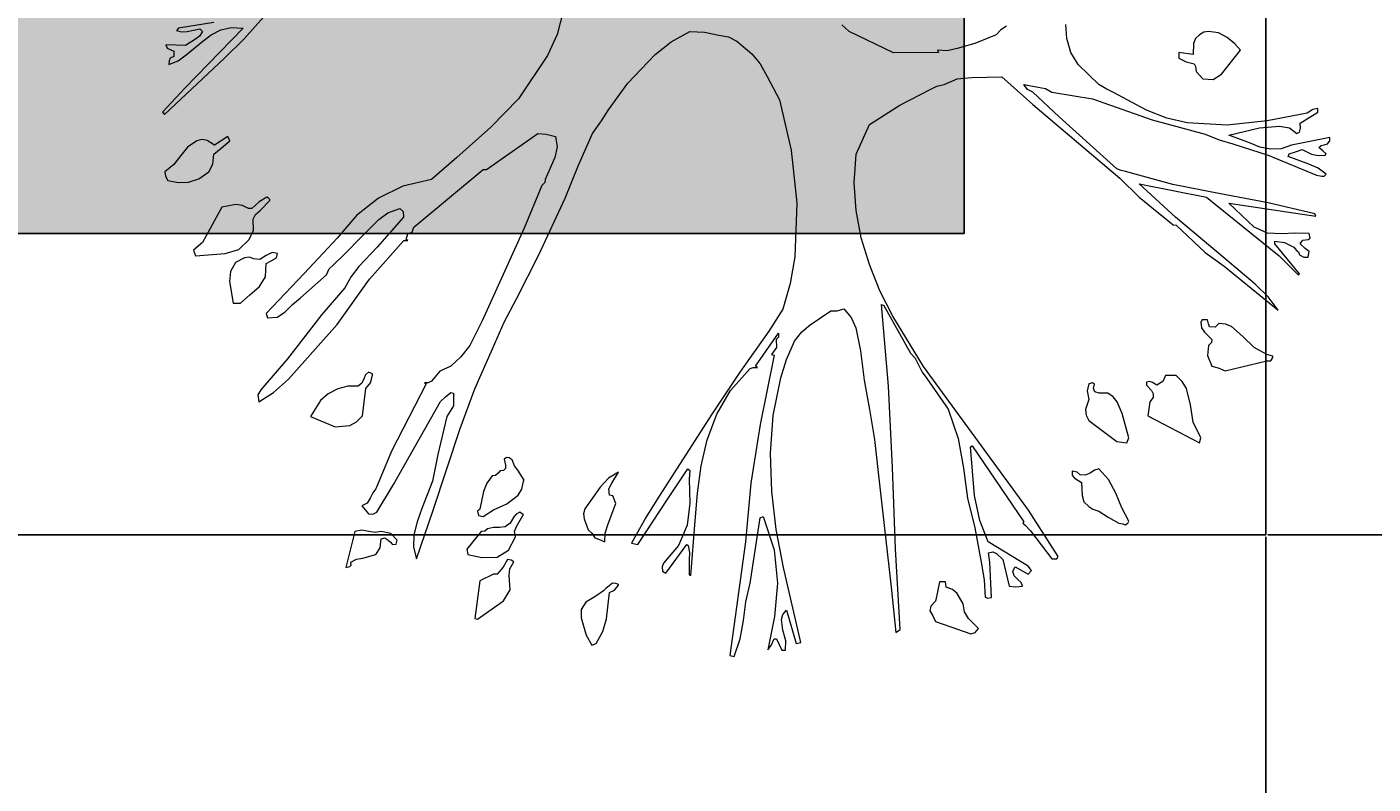
# Model space of a CAD drawing. Units: inches. Extents: x 84 to 1044, y -280 to 906.
# Tile 43 of 105: x 955 to 995, y -129 to -107. Entities that reach past the tile are written whole.
import ezdxf

# ---------------------------------------------------------------- set-up
doc = ezdxf.new("R2010")
doc.units = ezdxf.units.IN
for name, color, linetype, lineweight in [('A-ANNO-DIMS', 2, 'Continuous', 18), ('C-PROP', 7, 'Continuous', 25), ('L-PLNT', 114, 'Continuous', 15)]:
    doc.layers.add(name, color=color, linetype=linetype, lineweight=lineweight)
doc.layers.add('L-PLNT-PATT', color=9, linetype='Continuous', lineweight=9, true_color=0xafd9aa)
doc.styles.get("Standard").update_dxf_attribs({"font": 'arial.ttf'})
doc.dimstyles.get("Standard").update_dxf_attribs({"dimtxt": 0.18, "dimasz": 0.18, "dimexe": 0.18, "dimexo": 0.0625, "dimgap": 0.09, "dimtad": 0, "dimtih": 1, "dimtoh": 1, "dimdec": 4, "dimzin": 0, "dimdsep": 46, "dimtxsty": 'Standard', "dimcen": 0.09, "dimadec": 0, "dimazin": 0, "dimtfac": 1, "dimtdec": 4, "dimtofl": 0, "dimtmove": 0, "dimatfit": 3, "dimfxl": 1, "dimtolj": 1, "dimtzin": 0, "dimarcsym": 0})

# ---------------------------------------------------------------- blocks, each defined once
blk = doc.blocks.new('A$C37E508DF')
for p, q in [((0.9287, 0.7825), (0.936, 0.7542)), ((1.3151, 0.7487), (1.2919, 0.7752)), ((1.352, 0.7684), (1.3948, 0.7615)), ((0.1153, 0.7427), (0.1244, 0.7504)), ((0.1244, 0.7504), (0.1351, 0.7559)), ((0.1351, 0.7559), (0.1471, 0.7577)), ((0.1471, 0.7577), (0.1527, 0.7568)), ((0.1527, 0.7568), (0.1578, 0.7538)), ((0.1578, 0.7538), (0.1629, 0.7491)), ((0.3186, 0.7491), (0.3199, 0.7662)), ((0.3919, 0.7641), (0.3988, 0.7598)), ((0.3988, 0.7598), (0.4043, 0.7538)), ((0.4043, 0.7538), (0.4301, 0.7431)), ((0.5287, 0.7319), (0.5823, 0.7577)), ((0.5823, 0.7577), (0.5913, 0.7658)), ((0.7285, 0.7512), (0.7182, 0.7461)), ((0.7401, 0.7534), (0.7285, 0.7512)), ((0.7577, 0.7568), (0.7401, 0.7534)), ((0.7752, 0.7577), (0.7577, 0.7568)), ((0.798, 0.7452), (0.7752, 0.7577)), ((0.936, 0.7542), (0.9476, 0.7285)), ((1.3309, 0.7624), (1.3164, 0.7615)), ((1.3164, 0.7615), (1.3871, 0.6891)), ((1.3434, 0.7598), (1.3309, 0.7624)), ((1.355, 0.7538), (1.3434, 0.7598)), ((1.3653, 0.7461), (1.355, 0.7538)), ((1.3687, 0.7607), (1.3657, 0.7577)), ((1.3657, 0.7577), (1.3691, 0.7521)), ((1.3841, 0.7577), (1.3687, 0.7607)), ((1.3691, 0.7521), (1.3743, 0.7482)), ((1.3914, 0.7572), (1.3841, 0.7577)), ((1.397, 0.759), (1.3914, 0.7572)), ((1.3948, 0.7615), (1.397, 0.759)), ((0.1081, 0.7349), (0.1153, 0.7427)), ((0.1312, 0.7058), (0.1081, 0.7349)), ((0.1629, 0.7491), (0.1651, 0.7431)), ((0.1651, 0.7431), (0.1655, 0.7298)), ((0.3139, 0.7324), (0.3186, 0.7491)), ((0.4301, 0.7431), (0.4515, 0.7371)), ((0.4515, 0.7371), (0.4635, 0.7341)), ((0.4635, 0.7341), (0.4755, 0.7349)), ((0.4755, 0.7349), (0.4742, 0.7324)), ((0.7182, 0.7461), (0.7002, 0.7307)), ((0.8173, 0.7298), (0.798, 0.7452)), ((1.3391, 0.7255), (1.3151, 0.7487)), ((1.3854, 0.7294), (1.3653, 0.7461)), ((1.3743, 0.7482), (1.3863, 0.7405)), ((1.3863, 0.7405), (1.4099, 0.7414)), ((1.4086, 0.7375), (1.4004, 0.7337)), ((1.4099, 0.7414), (1.4086, 0.7375)), ((0.1646, 0.7186), (0.1629, 0.7152)), ((0.1741, 0.7208), (0.1646, 0.7186)), ((0.1655, 0.7298), (0.1831, 0.7324)), ((0.1831, 0.7255), (0.1741, 0.7208)), ((0.1831, 0.7324), (0.1831, 0.7255)), ((0.28, 0.6933), (0.3049, 0.7178)), ((0.3049, 0.7178), (0.3139, 0.7324)), ((0.4742, 0.7324), (0.5287, 0.7319)), ((0.6903, 0.7186), (0.6818, 0.7032)), ((0.7002, 0.7307), (0.6903, 0.7186)), ((0.8344, 0.7122), (0.8173, 0.7298)), ((0.9476, 0.7285), (0.9828, 0.6762)), ((1.4116, 0.6569), (1.3391, 0.7255)), ((1.3953, 0.7221), (1.3854, 0.7294)), ((1.4064, 0.7178), (1.3953, 0.7221)), ((1.4004, 0.7337), (1.4004, 0.7272)), ((1.4004, 0.7272), (1.4047, 0.7255)), ((1.4047, 0.7255), (1.406, 0.7221)), ((1.406, 0.7221), (1.4064, 0.7178)), ((0.1415, 0.6994), (0.1312, 0.7058)), ((0.1621, 0.7092), (0.1539, 0.7002)), ((0.1629, 0.7152), (0.1621, 0.7092)), ((0.3975, 0.7028), (0.3598, 0.6693)), ((0.4339, 0.7019), (0.3975, 0.7028)), ((0.4515, 0.7002), (0.4339, 0.7019)), ((0.6818, 0.7032), (0.6667, 0.6749)), ((0.8503, 0.6951), (0.8344, 0.7122)), ((0.1539, 0.7002), (0.1415, 0.6994)), ((0.262, 0.6839), (0.271, 0.6882)), ((0.271, 0.6882), (0.28, 0.6933)), ((0.3443, 0.6886), (0.337, 0.6843)), ((0.3533, 0.6903), (0.3443, 0.6886)), ((0.3709, 0.6933), (0.3533, 0.6903)), ((0.3598, 0.6843), (0.3662, 0.6873)), ((0.3662, 0.6873), (0.3709, 0.6933)), ((0.4674, 0.6933), (0.4515, 0.7002)), ((0.476, 0.6912), (0.4674, 0.6933)), ((0.4832, 0.6878), (0.476, 0.6912)), ((0.521, 0.6685), (0.4832, 0.6878)), ((0.8739, 0.6629), (0.8503, 0.6951)), ((1.3871, 0.6891), (1.4141, 0.6599)), ((0.2877, 0.6762), (0.2152, 0.6505)), ((0.2221, 0.6625), (0.262, 0.6839)), ((0.3598, 0.6693), (0.2543, 0.5797)), ((0.337, 0.6843), (0.2877, 0.6762)), ((0.328, 0.6543), (0.3598, 0.6843)), ((0.6667, 0.6749), (0.6526, 0.614)), ((0.9828, 0.6762), (1.0162, 0.6415)), ((0.0146, 0.6599), (0.0146, 0.6642)), ((0.0146, 0.6642), (0.0206, 0.6633)), ((0.036, 0.6466), (0.0146, 0.6599)), ((0.0206, 0.6633), (0.0274, 0.6586)), ((0.0274, 0.6586), (0.0759, 0.6492)), ((0.1728, 0.647), (0.1977, 0.6526)), ((0.1977, 0.6526), (0.2221, 0.6625)), ((0.2581, 0.5913), (0.328, 0.6543)), ((0.5578, 0.6449), (0.521, 0.6685)), ((0.8824, 0.6492), (0.8739, 0.6629)), ((1.4141, 0.6599), (1.4116, 0.6569)), ((0.0356, 0.6406), (0.036, 0.6466)), ((0.0369, 0.6355), (0.0356, 0.6406)), ((0.0489, 0.641), (0.0399, 0.6342)), ((0.0609, 0.6428), (0.0489, 0.641)), ((0.0853, 0.641), (0.0609, 0.6428)), ((0.0759, 0.6492), (0.1244, 0.644)), ((0.1226, 0.632), (0.0853, 0.641)), ((0.1244, 0.644), (0.1728, 0.647)), ((0.2152, 0.6505), (0.1509, 0.6333)), ((0.5737, 0.6089), (0.5578, 0.6449)), ((0.8932, 0.6342), (0.8824, 0.6492)), ((1.0162, 0.6415), (1.0574, 0.605)), ((0, 0.629), (0.0467, 0.62)), ((0, 0.6252), (0, 0.629)), ((0.003, 0.6213), (0, 0.6252)), ((0.0069, 0.6204), (0.003, 0.6213)), ((0.0107, 0.6196), (0.0069, 0.6204)), ((0.0399, 0.6342), (0.0369, 0.6355)), ((0.0467, 0.62), (0.0592, 0.6153)), ((0.1175, 0.6213), (0.0746, 0.6076)), ((0.0849, 0.6175), (0.0973, 0.6226)), ((0.0973, 0.6226), (0.1226, 0.632)), ((0.1342, 0.6265), (0.1175, 0.6213)), ((0.1509, 0.6333), (0.1342, 0.6265)), ((0.9103, 0.5956), (0.8932, 0.6342)), ((0.9382, 0.6303), (0.936, 0.6179)), ((0.9493, 0.6333), (0.9382, 0.6303)), ((0.9596, 0.6342), (0.9493, 0.6333)), ((1.0218, 0.5904), (0.9596, 0.6342)), ((1.3327, 0.6252), (1.3348, 0.6303)), ((1.343, 0.6162), (1.3327, 0.6252)), ((1.3348, 0.6303), (1.3511, 0.62)), ((1.3511, 0.62), (1.3601, 0.6256)), ((1.3601, 0.6256), (1.3661, 0.6269)), ((1.3661, 0.6269), (1.3725, 0.6252)), ((1.3725, 0.6252), (1.3837, 0.6175)), ((0.0047, 0.6093), (0.0086, 0.6132)), ((0.0056, 0.6076), (0.0047, 0.6093)), ((0.0141, 0.6072), (0.0056, 0.6076)), ((0.0086, 0.6132), (0.0133, 0.617)), ((0.0133, 0.617), (0.0107, 0.6196)), ((0.0223, 0.6089), (0.0141, 0.6072)), ((0.0746, 0.6076), (0.0163, 0.5836)), ((0.0334, 0.6145), (0.0223, 0.6089)), ((0.0257, 0.5969), (0.0506, 0.6063)), ((0.0416, 0.6119), (0.0334, 0.6145)), ((0.0493, 0.6093), (0.0416, 0.6119)), ((0.0506, 0.6063), (0.0493, 0.6093)), ((0.0592, 0.6153), (0.072, 0.6149)), ((0.072, 0.6149), (0.0849, 0.6175)), ((0.5763, 0.5741), (0.5737, 0.6089)), ((0.6526, 0.614), (0.6457, 0.5497)), ((0.936, 0.6179), (0.939, 0.605)), ((0.939, 0.605), (0.9506, 0.5784)), ((1.0574, 0.605), (1.0883, 0.5784)), ((1.352, 0.6089), (1.343, 0.6162)), ((1.3533, 0.5969), (1.352, 0.6089)), ((1.3837, 0.6175), (1.3918, 0.6072)), ((1.3918, 0.6072), (1.4004, 0.5964)), ((0.0047, 0.5849), (0.0141, 0.5921)), ((0.0141, 0.5921), (0.0257, 0.5969)), ((0.1904, 0.5724), (0.2474, 0.5879)), ((0.2474, 0.5879), (0.253, 0.5892)), ((0.253, 0.5892), (0.2581, 0.5913)), ((0.9262, 0.5557), (0.9103, 0.5956)), ((1.0256, 0.5904), (1.0218, 0.5904)), ((1.1097, 0.5205), (1.0256, 0.5904)), ((1.358, 0.5874), (1.3533, 0.5969)), ((1.37, 0.5789), (1.358, 0.5874)), ((1.4004, 0.5964), (1.4111, 0.5874)), ((1.4111, 0.5874), (1.4103, 0.5823)), ((0.0069, 0.5823), (0.0047, 0.5849)), ((0.0099, 0.5823), (0.0069, 0.5823)), ((0.0163, 0.5836), (0.0099, 0.5823)), ((0.1325, 0.5608), (0.1904, 0.5724)), ((0.2311, 0.5729), (0.1496, 0.557)), ((0.1869, 0.5325), (0.2311, 0.5729)), ((0.2543, 0.5797), (0.2311, 0.557)), ((0.5737, 0.5407), (0.5763, 0.5741)), ((0.9506, 0.5784), (0.951, 0.5746)), ((0.951, 0.5746), (0.9545, 0.5711)), ((0.9545, 0.5711), (0.9759, 0.5193)), ((1.0883, 0.5784), (1.123, 0.5703)), ((1.3824, 0.575), (1.37, 0.5789)), ((1.3953, 0.5746), (1.3824, 0.575)), ((1.4077, 0.5771), (1.3953, 0.5746)), ((1.4103, 0.5823), (1.4077, 0.5771)), ((0.1496, 0.557), (0.0613, 0.4858)), ((0.0746, 0.5501), (0.1325, 0.5608)), ((0.2311, 0.557), (0.1899, 0.5235)), ((0.9583, 0.4871), (0.9262, 0.5557)), ((1.123, 0.5703), (1.1526, 0.5557)), ((1.1526, 0.5557), (1.1792, 0.5347)), ((1.2842, 0.554), (1.2855, 0.5557)), ((1.2855, 0.5557), (1.2876, 0.557)), ((1.2876, 0.557), (1.2971, 0.551)), ((0.1226, 0.5497), (0.0171, 0.5338)), ((0.0184, 0.5368), (0.0746, 0.5501)), ((0.0917, 0.5205), (0.1226, 0.5497)), ((0.5677, 0.5077), (0.5737, 0.5407)), ((0.6457, 0.5497), (0.6483, 0.4845)), ((1.1226, 0.5394), (1.1221, 0.5325)), ((1.1268, 0.5433), (1.1226, 0.5394)), ((1.141, 0.5377), (1.1268, 0.5433)), ((1.2842, 0.5527), (1.2842, 0.554)), ((1.2958, 0.5407), (1.2842, 0.5527)), ((1.3014, 0.536), (1.2958, 0.5407)), ((1.2971, 0.551), (1.3057, 0.5433)), ((1.3057, 0.5433), (1.3099, 0.5433)), ((1.3099, 0.5433), (1.3172, 0.5467)), ((1.3172, 0.5467), (1.3254, 0.548)), ((1.3254, 0.548), (1.3421, 0.5446)), ((1.3421, 0.5446), (1.3657, 0.5021)), ((0.0171, 0.5338), (0.0184, 0.5368)), ((0.1269, 0.482), (0.1869, 0.5325)), ((0.1861, 0.5231), (0.1509, 0.4897)), ((0.1899, 0.5235), (0.1861, 0.5231)), ((1.1221, 0.5325), (1.1539, 0.4961)), ((1.1521, 0.5296), (1.141, 0.5377)), ((1.1706, 0.5111), (1.1521, 0.5296)), ((1.1792, 0.5347), (1.2027, 0.5072)), ((1.3044, 0.53), (1.3014, 0.536)), ((1.3039, 0.5167), (1.3044, 0.53)), ((0.024, 0.5072), (0.0253, 0.5128)), ((0.0262, 0.5055), (0.024, 0.5072)), ((0.0253, 0.5128), (0.042, 0.5133)), ((0.0326, 0.5047), (0.0262, 0.5055)), ((0.042, 0.5133), (0.0587, 0.5124)), ((0.0587, 0.5124), (0.0755, 0.5133)), ((0.0755, 0.5133), (0.0917, 0.5205)), ((0.5578, 0.4751), (0.5677, 0.5077)), ((0.9759, 0.5193), (1.0269, 0.4069)), ((1.1118, 0.5145), (1.1097, 0.5205)), ((1.117, 0.5124), (1.1118, 0.5145)), ((1.1191, 0.5055), (1.117, 0.5124)), ((1.117, 0.5042), (1.1191, 0.5055)), ((1.1955, 0.4858), (1.1706, 0.5111)), ((1.2027, 0.5072), (1.2426, 0.4644)), ((1.3091, 0.5055), (1.3039, 0.5167)), ((1.3215, 0.4935), (1.3091, 0.5055)), ((0.0253, 0.491), (0.03, 0.4948)), ((0.0262, 0.4841), (0.0253, 0.491)), ((0.03, 0.4948), (0.036, 0.5004)), ((0.036, 0.5004), (0.0326, 0.5047)), ((0.0369, 0.4639), (0.0669, 0.5004)), ((0.0382, 0.4905), (0.0369, 0.4871)), ((0.0403, 0.4922), (0.0382, 0.4905)), ((0.0437, 0.4961), (0.0403, 0.4922)), ((0.0549, 0.5021), (0.0437, 0.4961)), ((0.0669, 0.5034), (0.0549, 0.5021)), ((0.0669, 0.5004), (0.0669, 0.5034)), ((0.1509, 0.4897), (0.1282, 0.4734)), ((1.1217, 0.5042), (1.117, 0.5042)), ((1.1633, 0.4575), (1.1217, 0.5042)), ((1.1539, 0.4961), (1.1762, 0.4729)), ((1.2748, 0.4884), (1.2812, 0.4897)), ((1.2812, 0.4897), (1.2885, 0.4862)), ((1.3382, 0.4884), (1.3215, 0.4935)), ((1.3657, 0.5021), (1.3764, 0.4927)), ((1.3764, 0.4927), (1.3743, 0.4858)), ((0.0317, 0.4841), (0.0262, 0.4841)), ((0.0369, 0.4871), (0.0317, 0.4841)), ((0.0613, 0.4858), (0.0386, 0.4627)), ((0.1282, 0.4734), (0.0626, 0.4198)), ((0.0905, 0.4515), (0.1269, 0.482)), ((0.545, 0.4434), (0.5578, 0.4751)), ((0.6483, 0.4845), (0.6539, 0.4524)), ((0.9853, 0.4335), (0.9583, 0.4871)), ((1.1762, 0.4729), (1.1856, 0.4605)), ((1.207, 0.4747), (1.1955, 0.4858)), ((1.2122, 0.47), (1.207, 0.4747)), ((1.2761, 0.4832), (1.2748, 0.4884)), ((1.2825, 0.4798), (1.2761, 0.4832)), ((1.2885, 0.4764), (1.2825, 0.4798)), ((1.2885, 0.4862), (1.2962, 0.4815)), ((1.2894, 0.4601), (1.2885, 0.4764)), ((1.2962, 0.4815), (1.3039, 0.482)), ((1.3039, 0.482), (1.3087, 0.4841)), ((1.3087, 0.4841), (1.3147, 0.4832)), ((1.3147, 0.4832), (1.3258, 0.4777)), ((1.3258, 0.4777), (1.3318, 0.4669)), ((1.3743, 0.4858), (1.3382, 0.4884)), ((0.0386, 0.4627), (0.0369, 0.4639)), ((1.2027, 0.4026), (1.1633, 0.4575)), ((1.1856, 0.4605), (1.1933, 0.4468)), ((1.2156, 0.4627), (1.2122, 0.47)), ((1.2469, 0.4348), (1.2156, 0.4627)), ((1.2426, 0.4644), (1.2885, 0.4159)), ((1.2967, 0.4485), (1.2894, 0.4601)), ((1.3318, 0.4669), (1.3331, 0.4545)), ((0.0746, 0.4361), (0.0905, 0.4515)), ((0.5295, 0.4125), (0.545, 0.4434)), ((0.6539, 0.4524), (0.6625, 0.4211)), ((1.1933, 0.4468), (1.2212, 0.4146)), ((1.3082, 0.4386), (1.2967, 0.4485)), ((1.3331, 0.4545), (1.3284, 0.4284)), ((0.0626, 0.4198), (0.0746, 0.4361)), ((0.5403, 0.4254), (0.5081, 0.3679)), ((0.5347, 0.3276), (0.5433, 0.4266)), ((0.5433, 0.4266), (0.5403, 0.4254)), ((1.0003, 0.4052), (0.9853, 0.4335)), ((1.2568, 0.4266), (1.2469, 0.4348)), ((1.2658, 0.4176), (1.2568, 0.4266)), ((1.3198, 0.4284), (1.3082, 0.4386)), ((1.3284, 0.4284), (1.3198, 0.4284)), ((0.1471, 0.4035), (0.1484, 0.4082)), ((0.1484, 0.4082), (0.1548, 0.4082)), ((0.1548, 0.4082), (0.1565, 0.4052)), ((0.4922, 0.3516), (0.5295, 0.4125)), ((0.5797, 0.4112), (0.5741, 0.3983)), ((0.5887, 0.4215), (0.5797, 0.4112)), ((0.5969, 0.4189), (0.5887, 0.4215)), ((0.6046, 0.4189), (0.5969, 0.4189)), ((0.6295, 0.4022), (0.6046, 0.4189)), ((0.6625, 0.4211), (0.6796, 0.3945)), ((1.2212, 0.4146), (1.2628, 0.361)), ((1.2752, 0.4116), (1.2658, 0.4176)), ((1.2868, 0.4108), (1.2752, 0.4116)), ((1.2885, 0.4159), (1.2868, 0.4108)), ((0.1055, 0.388), (0.1192, 0.4001)), ((0.1192, 0.4001), (0.1265, 0.4031)), ((0.1265, 0.4031), (0.1346, 0.4039)), ((0.1346, 0.4039), (0.1389, 0.3992)), ((0.1389, 0.3992), (0.1458, 0.3996)), ((0.1518, 0.3932), (0.1432, 0.3842)), ((0.1458, 0.3996), (0.1471, 0.4035)), ((0.1556, 0.3983), (0.1518, 0.3932)), ((0.1565, 0.4052), (0.1556, 0.3983)), ((0.5741, 0.3983), (0.5686, 0.3705)), ((0.6397, 0.3936), (0.6295, 0.4022)), ((0.6487, 0.3825), (0.6397, 0.3936)), ((0.6959, 0.352), (0.668, 0.3919)), ((0.668, 0.3919), (0.668, 0.3872)), ((0.6796, 0.3945), (0.7148, 0.3447)), ((1.0145, 0.373), (1.0003, 0.4052)), ((1.0269, 0.4069), (1.0419, 0.3769)), ((1.2289, 0.373), (1.2027, 0.4026)), ((0.0917, 0.3748), (0.1055, 0.388)), ((0.1432, 0.3842), (0.1436, 0.3808)), ((0.1436, 0.3808), (0.1471, 0.3769)), ((0.1471, 0.3769), (0.1484, 0.3649)), ((0.6582, 0.3602), (0.6487, 0.3825)), ((0.668, 0.3872), (0.6706, 0.3842)), ((0.6706, 0.3842), (0.6702, 0.3748)), ((1.0419, 0.3769), (1.0527, 0.3632)), ((0.069, 0.364), (0.0763, 0.3662)), ((0.069, 0.3627), (0.069, 0.364)), ((0.0716, 0.3585), (0.069, 0.3627)), ((0.0763, 0.3662), (0.0917, 0.3748)), ((0.1484, 0.3649), (0.1432, 0.352)), ((0.5025, 0.3619), (0.4982, 0.3537)), ((0.5081, 0.3679), (0.5025, 0.3619)), ((0.5686, 0.3705), (0.5643, 0.3349)), ((0.665, 0.3379), (0.6582, 0.3602)), ((0.6702, 0.3748), (0.6762, 0.3662)), ((0.6762, 0.3662), (0.6732, 0.3653)), ((0.6732, 0.3653), (0.6903, 0.2813)), ((1.0359, 0.3246), (1.0145, 0.373)), ((1.0527, 0.3632), (1.0647, 0.352)), ((1.2615, 0.3362), (1.2289, 0.373)), ((1.2628, 0.361), (1.2949, 0.3233)), ((0.0763, 0.3585), (0.0716, 0.3585)), ((0.1269, 0.3464), (0.0763, 0.3585)), ((0.1355, 0.3499), (0.1269, 0.3464)), ((0.1432, 0.352), (0.1355, 0.3499)), ((0.4065, 0.2345), (0.4922, 0.3516)), ((0.4939, 0.3447), (0.4884, 0.337)), ((0.4982, 0.3537), (0.4939, 0.3447)), ((0.6933, 0.3503), (0.6959, 0.352)), ((0.6985, 0.3503), (0.6933, 0.3503)), ((0.7023, 0.349), (0.6985, 0.3503)), ((0.7259, 0.3224), (0.7023, 0.349)), ((0.7148, 0.3447), (0.7487, 0.2937)), ((1.0647, 0.352), (1.078, 0.346)), ((1.078, 0.346), (1.0883, 0.334)), ((1.1599, 0.3426), (1.1646, 0.3447)), ((1.1599, 0.3413), (1.1599, 0.3426)), ((1.1646, 0.3447), (1.168, 0.3417)), ((0.1737, 0.325), (0.1788, 0.3336)), ((0.1788, 0.3336), (0.1861, 0.3409)), ((0.1861, 0.3409), (0.199, 0.3409)), ((0.199, 0.3409), (0.2024, 0.3336)), ((0.2024, 0.3336), (0.2097, 0.3289)), ((0.2097, 0.3289), (0.2148, 0.3323)), ((0.2148, 0.3323), (0.2182, 0.3336)), ((0.2221, 0.3289), (0.2161, 0.3224)), ((0.2182, 0.3336), (0.2221, 0.3327)), ((0.2221, 0.3327), (0.2221, 0.3289)), ((0.2851, 0.3302), (0.2877, 0.3319)), ((0.2864, 0.325), (0.2851, 0.3302)), ((0.2877, 0.3319), (0.292, 0.3306)), ((0.292, 0.3306), (0.2941, 0.322)), ((0.4884, 0.337), (0.4622, 0.2997)), ((0.53, 0.229), (0.5347, 0.3276)), ((0.5643, 0.3349), (0.5578, 0.2993)), ((0.6745, 0.2924), (0.665, 0.3379)), ((1.0883, 0.334), (1.0921, 0.3319)), ((1.0921, 0.3319), (1.0968, 0.3319)), ((1.0968, 0.3319), (1.0947, 0.3306)), ((1.0947, 0.3306), (1.1367, 0.2491)), ((1.162, 0.3319), (1.1599, 0.3413)), ((1.1676, 0.325), (1.162, 0.3319)), ((1.168, 0.3417), (1.1702, 0.3366)), ((1.1702, 0.3366), (1.1727, 0.3314)), ((1.1727, 0.3314), (1.177, 0.3276)), ((1.177, 0.3276), (1.1895, 0.3276)), ((1.1895, 0.3276), (1.2019, 0.3246)), ((1.2795, 0.3199), (1.2615, 0.3362)), ((0.1689, 0.3053), (0.1737, 0.325)), ((0.2161, 0.3224), (0.214, 0.3186)), ((0.214, 0.3186), (0.214, 0.3139)), ((0.214, 0.3139), (0.2182, 0.3087)), ((0.2577, 0.3087), (0.2624, 0.3147)), ((0.2624, 0.3147), (0.2689, 0.3194)), ((0.2689, 0.3194), (0.2796, 0.3194)), ((0.2796, 0.3194), (0.2847, 0.3211)), ((0.2847, 0.3211), (0.2864, 0.325)), ((0.2941, 0.322), (0.292, 0.3117)), ((0.292, 0.3117), (0.2959, 0.2993)), ((0.7427, 0.2937), (0.7259, 0.3224)), ((1.0535, 0.2766), (1.0359, 0.3246)), ((1.0647, 0.3199), (1.0617, 0.3194)), ((1.0617, 0.3194), (1.0617, 0.304)), ((1.0711, 0.3147), (1.0647, 0.3199)), ((1.0775, 0.3092), (1.0711, 0.3147)), ((1.1719, 0.292), (1.1676, 0.325)), ((1.2019, 0.3246), (1.2135, 0.3186)), ((1.2135, 0.3186), (1.2225, 0.3104)), ((1.2225, 0.3104), (1.2349, 0.2911)), ((1.2975, 0.3087), (1.2795, 0.3199)), ((1.2949, 0.3233), (1.2988, 0.3173)), ((1.2988, 0.3173), (1.2975, 0.3087)), ((0.1655, 0.2843), (0.1689, 0.3053)), ((0.2182, 0.3087), (0.2204, 0.292)), ((0.2436, 0.265), (0.2517, 0.2946)), ((0.2517, 0.2946), (0.2577, 0.3087)), ((0.2959, 0.2993), (0.2954, 0.2928)), ((0.4622, 0.2997), (0.4502, 0.2645)), ((0.5578, 0.2993), (0.5518, 0.2633)), ((0.7542, 0.2628), (0.7427, 0.2937)), ((0.7487, 0.2937), (0.8151, 0.1899)), ((1.0617, 0.304), (1.0698, 0.2911)), ((1.1341, 0.2084), (1.0775, 0.3092)), ((0.1565, 0.265), (0.1655, 0.2843)), ((0.2204, 0.292), (0.1578, 0.259)), ((0.292, 0.286), (0.2581, 0.2607)), ((0.2954, 0.2928), (0.292, 0.286)), ((0.6775, 0.2465), (0.6745, 0.2924)), ((0.6903, 0.2813), (0.7015, 0.2101)), ((1.0698, 0.2911), (1.0805, 0.2448)), ((1.1792, 0.2847), (1.1719, 0.292)), ((1.1873, 0.28), (1.1792, 0.2847)), ((1.2049, 0.2783), (1.1873, 0.28)), ((1.2349, 0.2911), (1.2049, 0.2783)), ((0.1578, 0.259), (0.1565, 0.265)), ((0.2461, 0.259), (0.2436, 0.265)), ((0.4502, 0.2645), (0.4438, 0.2285)), ((0.5518, 0.2633), (0.5475, 0.2268)), ((0.7615, 0.2311), (0.7542, 0.2628)), ((1.0861, 0.1775), (1.0535, 0.2766)), ((0.2581, 0.2607), (0.2461, 0.259)), ((0.4335, 0.2556), (0.3709, 0.1634)), ((0.4305, 0.1951), (0.4352, 0.2543)), ((0.4352, 0.2543), (0.4335, 0.2556)), ((0.6758, 0.2002), (0.6775, 0.2465)), ((1.0805, 0.2448), (1.087, 0.2127)), ((1.1367, 0.2491), (1.1556, 0.2032)), ((0.3649, 0.1775), (0.4065, 0.2345)), ((0.4438, 0.2285), (0.4391, 0.1921)), ((0.5261, 0.1308), (0.53, 0.229)), ((0.7662, 0.1981), (0.7615, 0.2311)), ((0.9836, 0.226), (0.9879, 0.2311)), ((0.9879, 0.2311), (0.9905, 0.2384)), ((0.9905, 0.2384), (0.9943, 0.241)), ((0.9943, 0.241), (0.9973, 0.2414)), ((0.9973, 0.2414), (1.0003, 0.2393)), ((1.0003, 0.2393), (0.9986, 0.232)), ((0.9986, 0.232), (0.9986, 0.2281)), ((0.2594, 0.1981), (0.268, 0.2148)), ((0.268, 0.2148), (0.28, 0.2277)), ((0.28, 0.2277), (0.2851, 0.226)), ((0.2851, 0.226), (0.2903, 0.2225)), ((0.2903, 0.2225), (0.2963, 0.22)), ((0.2963, 0.22), (0.3027, 0.2204)), ((0.3096, 0.2165), (0.301, 0.211)), ((0.3027, 0.2204), (0.3061, 0.2234)), ((0.3061, 0.2234), (0.3122, 0.2247)), ((0.3122, 0.22), (0.3096, 0.2165)), ((0.3122, 0.2247), (0.3122, 0.22)), ((0.5475, 0.2268), (0.5313, 0.084)), ((0.7778, 0.2277), (0.7752, 0.2255)), ((0.7752, 0.2255), (0.7761, 0.2152)), ((0.7761, 0.2152), (0.7752, 0.1861)), ((0.8018, 0.1912), (0.7778, 0.2277)), ((0.8619, 0.2234), (0.8739, 0.2161)), ((0.87, 0.2101), (0.8619, 0.2234)), ((0.8739, 0.2161), (0.8841, 0.2054)), ((0.9759, 0.214), (0.9836, 0.226)), ((0.9768, 0.2127), (0.9759, 0.214)), ((0.9789, 0.2028), (0.9768, 0.2127)), ((0.9986, 0.2281), (1.0012, 0.2255)), ((1.0012, 0.2255), (1.0051, 0.2251)), ((1.0051, 0.2251), (1.0076, 0.2225)), ((1.0076, 0.2225), (1.0106, 0.2195)), ((1.0106, 0.2195), (1.0149, 0.2191)), ((1.0149, 0.2191), (1.0214, 0.2101)), ((1.087, 0.2127), (1.0998, 0.1797)), ((0.2521, 0.1805), (0.2594, 0.1981)), ((0.301, 0.211), (0.3002, 0.1951)), ((0.6706, 0.1539), (0.6758, 0.2002)), ((0.7015, 0.2101), (0.7079, 0.1389)), ((0.7688, 0.1646), (0.7662, 0.1981)), ((0.8734, 0.2032), (0.87, 0.2101)), ((0.8726, 0.1955), (0.8734, 0.2032)), ((0.8841, 0.2054), (0.9026, 0.1792)), ((0.9832, 0.1955), (0.9789, 0.2028)), ((1.0214, 0.2101), (1.0252, 0.2002)), ((1.0252, 0.2002), (1.0295, 0.1788)), ((1.1543, 0.1749), (1.1341, 0.2084)), ((1.1556, 0.2032), (1.1594, 0.1985)), ((1.1594, 0.1985), (1.1624, 0.1921)), ((0.2436, 0.1642), (0.2521, 0.1805)), ((0.292, 0.1818), (0.2873, 0.1788)), ((0.298, 0.1874), (0.292, 0.1818)), ((0.3002, 0.1951), (0.298, 0.1874)), ((0.4241, 0.1651), (0.4305, 0.1951)), ((0.4391, 0.1921), (0.4301, 0.1561)), ((0.7752, 0.1861), (0.7787, 0.1591)), ((0.8383, 0.1359), (0.8018, 0.1912)), ((0.8151, 0.1899), (0.8288, 0.1685)), ((0.8649, 0.1857), (0.8687, 0.1947)), ((0.8743, 0.1608), (0.8649, 0.1857)), ((0.8687, 0.1947), (0.8726, 0.1955)), ((0.9969, 0.1852), (0.9832, 0.1955)), ((1.0132, 0.1779), (0.9969, 0.1852)), ((1.0998, 0.1797), (1.1058, 0.1634)), ((1.1624, 0.1921), (1.1663, 0.1861)), ((1.1727, 0.1827), (1.1646, 0.1732)), ((1.1663, 0.1861), (1.1727, 0.1827)), ((0.2448, 0.1616), (0.2436, 0.1642)), ((0.2684, 0.1689), (0.2556, 0.1616)), ((0.28, 0.1762), (0.2684, 0.1689)), ((0.2873, 0.1788), (0.28, 0.1762)), ((0.3293, 0.1213), (0.3649, 0.1775)), ((0.3709, 0.1634), (0.3718, 0.1616)), ((0.4138, 0.1389), (0.4241, 0.1651)), ((0.6865, 0.1698), (0.6732, 0.1295)), ((0.6903, 0.1681), (0.6865, 0.1698)), ((0.7023, 0.0892), (0.6903, 0.1681)), ((0.774, 0.0982), (0.7688, 0.1646)), ((0.8288, 0.1685), (0.846, 0.1376)), ((0.9035, 0.1668), (0.8983, 0.1535)), ((0.9026, 0.1792), (0.9043, 0.1732)), ((0.9043, 0.1732), (0.9035, 0.1668)), ((0.9768, 0.1719), (0.9811, 0.1749)), ((0.9776, 0.1711), (0.9768, 0.1719)), ((0.9853, 0.1578), (0.9776, 0.1711)), ((0.9811, 0.1749), (0.9858, 0.1728)), ((0.9858, 0.1728), (0.9884, 0.1694)), ((0.9884, 0.1694), (0.9931, 0.1616)), ((1.0256, 0.1698), (1.0132, 0.1779)), ((1.0312, 0.1711), (1.0256, 0.1698)), ((1.0295, 0.1788), (1.0325, 0.1762)), ((1.0325, 0.1762), (1.0312, 0.1711)), ((1.1063, 0.1183), (1.0861, 0.1775)), ((1.1058, 0.1634), (1.1097, 0.1475)), ((1.1594, 0.1728), (1.1543, 0.1749)), ((1.1646, 0.1732), (1.1594, 0.1728)), ((0.2478, 0.1599), (0.2448, 0.1616)), ((0.2508, 0.1608), (0.2478, 0.1599)), ((0.2556, 0.1616), (0.2508, 0.1608)), ((0.3628, 0.1526), (0.337, 0.1183)), ((0.3692, 0.1591), (0.3628, 0.1526)), ((0.3718, 0.1616), (0.3692, 0.1591)), ((0.4301, 0.1561), (0.4224, 0.1145)), ((0.662, 0.108), (0.6706, 0.1539)), ((0.7787, 0.1591), (0.789, 0.1346)), ((0.8777, 0.1496), (0.8743, 0.1608)), ((0.8781, 0.1389), (0.8777, 0.1496)), ((0.894, 0.1496), (0.8902, 0.1441)), ((0.8983, 0.1535), (0.894, 0.1496)), ((0.9879, 0.1518), (0.9853, 0.1578)), ((0.9866, 0.1453), (0.9879, 0.1518)), ((0.9931, 0.1616), (0.9991, 0.1574)), ((0.9991, 0.1574), (1.0059, 0.1565)), ((1.0059, 0.1565), (1.0132, 0.1565)), ((1.0132, 0.1565), (1.0205, 0.1548)), ((1.0205, 0.1548), (1.0235, 0.1522)), ((1.0235, 0.1522), (1.0282, 0.1518)), ((1.0282, 0.1518), (1.0454, 0.1303)), ((1.1097, 0.1475), (1.1101, 0.1325)), ((1.1298, 0.1411), (1.1376, 0.1492)), ((1.1376, 0.1492), (1.1491, 0.1518)), ((1.1491, 0.1518), (1.1564, 0.1505)), ((1.1564, 0.1505), (1.1642, 0.1518)), ((1.1642, 0.1518), (1.1727, 0.1531)), ((1.1727, 0.1531), (1.1813, 0.1518)), ((1.1813, 0.1518), (1.192, 0.108)), ((0.3653, 0.1098), (0.4138, 0.1389)), ((0.5205, 0.033), (0.5261, 0.1308)), ((0.7079, 0.1389), (0.7268, 0.0013)), ((0.7774, 0.1346), (0.7757, 0.1261)), ((0.7791, 0.1359), (0.7774, 0.1346)), ((0.8044, 0.1012), (0.7791, 0.1359)), ((0.789, 0.1346), (0.8074, 0.1132)), ((0.846, 0.1376), (0.8383, 0.1359)), ((0.8846, 0.1419), (0.8781, 0.1389)), ((0.8902, 0.1441), (0.8846, 0.1419)), ((0.9948, 0.1291), (0.9866, 0.1453)), ((1.1101, 0.1325), (1.1063, 0.1183)), ((1.1311, 0.1364), (1.1298, 0.1411)), ((1.1354, 0.1359), (1.1311, 0.1364)), ((1.1384, 0.1389), (1.1354, 0.1359)), ((1.1423, 0.1423), (1.1384, 0.1389)), ((1.1449, 0.1441), (1.1423, 0.1423)), ((1.1491, 0.1428), (1.1449, 0.1441)), ((1.1504, 0.132), (1.1491, 0.1428)), ((1.1556, 0.1239), (1.1504, 0.132)), ((0.3306, 0.1183), (0.3293, 0.1213)), ((0.337, 0.1183), (0.3306, 0.1183)), ((0.3962, 0.1175), (0.3885, 0.0853)), ((0.4039, 0.1248), (0.3962, 0.1175)), ((0.4082, 0.1269), (0.4039, 0.1248)), ((0.4134, 0.1256), (0.4082, 0.1269)), ((0.4099, 0.0716), (0.4121, 0.1145)), ((0.4121, 0.1145), (0.4134, 0.1256)), ((0.4224, 0.1145), (0.4189, 0.093)), ((0.6732, 0.1295), (0.6693, 0.0892)), ((0.7757, 0.1261), (0.7761, 0.117)), ((0.7761, 0.117), (0.7761, 0.099)), ((0.9884, 0.1149), (0.9918, 0.117)), ((0.9935, 0.1063), (0.9884, 0.1149)), ((0.9918, 0.117), (0.9961, 0.1175)), ((1.0089, 0.1205), (0.9948, 0.1291)), ((0.9961, 0.1175), (1.0016, 0.1085)), ((1.0274, 0.12), (1.0089, 0.1205)), ((1.0441, 0.1239), (1.0274, 0.12)), ((1.0454, 0.1303), (1.0441, 0.1239)), ((1.1714, 0.1192), (1.1556, 0.1239)), ((1.1792, 0.1179), (1.1714, 0.1192)), ((1.186, 0.1145), (1.1792, 0.1179)), ((1.1856, 0.111), (1.186, 0.1145)), ((0.3615, 0.1042), (0.3653, 0.1098)), ((0.3653, 0.0999), (0.3615, 0.1042)), ((0.3812, 0.1089), (0.3653, 0.0999)), ((0.3842, 0.1037), (0.3812, 0.1089)), ((0.3825, 0.0978), (0.3842, 0.1037)), ((0.641, 0.0172), (0.662, 0.108)), ((0.7761, 0.099), (0.774, 0.0982)), ((0.8083, 0.1037), (0.8044, 0.1012)), ((0.8074, 0.1132), (0.8087, 0.1089)), ((0.8087, 0.1089), (0.8083, 0.1037)), ((0.9931, 0.081), (0.9943, 0.0982)), ((0.9943, 0.0982), (0.9935, 0.1063)), ((1.0016, 0.1085), (1.0089, 0.0999)), ((1.0089, 0.0999), (1.0132, 0.0999)), ((1.0132, 0.0999), (1.0295, 0.0917)), ((1.1873, 0.1093), (1.1856, 0.111)), ((1.192, 0.108), (1.1873, 0.1093)), ((0.3722, 0.0853), (0.3739, 0.09)), ((0.3808, 0.0845), (0.3722, 0.0853)), ((0.3739, 0.09), (0.3782, 0.0935)), ((0.3782, 0.0935), (0.3825, 0.0978)), ((0.3885, 0.0853), (0.3808, 0.0845)), ((0.4189, 0.093), (0.4176, 0.072)), ((0.4571, 0.0815), (0.4648, 0.084)), ((0.4648, 0.084), (0.4657, 0.0905)), ((0.4657, 0.0905), (0.473, 0.0905)), ((0.473, 0.0905), (0.476, 0.0746)), ((0.5313, 0.084), (0.5257, 0.0291)), ((0.6693, 0.0892), (0.6728, 0.0484)), ((0.7075, 0.0665), (0.7023, 0.0892)), ((0.8619, 0.0875), (0.8649, 0.0887)), ((0.8619, 0.0866), (0.8619, 0.0875)), ((0.8666, 0.0806), (0.8619, 0.0866)), ((0.8649, 0.0887), (0.8691, 0.0892)), ((0.8691, 0.0892), (0.8769, 0.0827)), ((0.8769, 0.0827), (0.8799, 0.0797)), ((1.0295, 0.0917), (1.0359, 0.0463)), ((0.4142, 0.0707), (0.4099, 0.0716)), ((0.4176, 0.072), (0.4142, 0.0707)), ((0.4442, 0.0639), (0.4515, 0.0763)), ((0.4515, 0.0763), (0.4571, 0.0815)), ((0.476, 0.0746), (0.4777, 0.0673)), ((0.4777, 0.0673), (0.4832, 0.0613)), ((0.7105, 0.0437), (0.7075, 0.0665)), ((0.8726, 0.0776), (0.8666, 0.0806)), ((0.8764, 0.0459), (0.8726, 0.0776)), ((0.8799, 0.0797), (0.8893, 0.0733)), ((0.8893, 0.0733), (0.9013, 0.066)), ((0.9013, 0.066), (0.9069, 0.057)), ((1.0012, 0.0677), (0.9931, 0.081)), ((1.0325, 0.0454), (1.0012, 0.0677)), ((0.4378, 0.0463), (0.4425, 0.0544)), ((0.4425, 0.0544), (0.4442, 0.0639)), ((0.4811, 0.0493), (0.4777, 0.0424)), ((0.4845, 0.0553), (0.4811, 0.0493)), ((0.4832, 0.0613), (0.4845, 0.0553)), ((0.6582, 0.0562), (0.6466, 0.0159)), ((0.6625, 0.051), (0.6582, 0.0562)), ((0.6642, 0.045), (0.6625, 0.051)), ((0.9069, 0.057), (0.9069, 0.0471)), ((0.4258, 0.0339), (0.4378, 0.0463)), ((0.4296, 0.0291), (0.4258, 0.0339)), ((0.4777, 0.0424), (0.4348, 0.0274)), ((0.5257, 0.0291), (0.5205, 0.033)), ((0.6625, 0.0321), (0.6642, 0.045)), ((0.6728, 0.0484), (0.6809, 0.0082)), ((0.7144, 0.0214), (0.7105, 0.0437)), ((0.8807, 0.0304), (0.8764, 0.0459)), ((0.9069, 0.0471), (0.9009, 0.0261)), ((1.0359, 0.0463), (1.0325, 0.0454)), ((0.4348, 0.0274), (0.4296, 0.0291)), ((0.6466, 0.0159), (0.641, 0.0172)), ((0.659, 0.0193), (0.6625, 0.0321)), ((0.6595, 0.0077), (0.659, 0.0193)), ((0.6702, 0.0214), (0.6637, 0.0077)), ((0.6732, 0.0214), (0.6702, 0.0214)), ((0.6766, 0.0133), (0.6732, 0.0214)), ((0.7216, 0), (0.7144, 0.0214)), ((0.8889, 0.0159), (0.8807, 0.0304)), ((0.9009, 0.0261), (0.894, 0.0137)), ((0.6637, 0.0077), (0.6595, 0.0077)), ((0.6809, 0.0082), (0.6766, 0.0133)), ((0.7268, 0.0013), (0.7216, 0)), ((0.894, 0.0137), (0.8889, 0.0159))]:
    blk.add_line(p, q)
blk = doc.blocks.new('*D60')
at = {"layer": 'A-ANNO-DIMS', "color": 0, "lineweight": -2, "transparency": 16777216}
for p, q in [((134.179, -121.942), (134.179, -180.64)), ((992.074, -121.942), (992.074, -180.64)), ((134.359, -180.46), (562.733, -180.46)), ((991.894, -180.46), (563.521, -180.46))]:
    blk.add_line(p, q, dxfattribs=at)
at = {"layer": 'A-ANNO-DIMS', "color": 0, "transparency": 16777216}
for points in [[(134.359, -180.43), (134.359, -180.49), (134.179, -180.46)], [(991.894, -180.43), (991.894, -180.49), (992.074, -180.46)]]:
    blk.add_solid(points, dxfattribs=at)
at = {"layer": 'Defpoints', "color": 0, "transparency": 16777216}
for p in [(134.179, -121.88), (992.074, -121.88), (992.074, -180.46)]:
    blk.add_point(p, dxfattribs=at)
at = {"layer": 'A-ANNO-DIMS', "color": 0, "transparency": 16777216, "insert": (563.127, -180.46), "char_height": 0.18, "attachment_point": 5}
blk.add_mtext('\\A1;857.9', dxfattribs=at)
blk = doc.blocks.new('*D70')
at = {"layer": 'A-ANNO-DIMS', "color": 0, "lineweight": -2, "transparency": 16777216}
for p, q in [((983.136, -64.88), (1043.768, -64.88)), ((1043.588, -65.06), (1043.588, -93.198)), ((1043.588, -121.7), (1043.588, -93.561)), ((992.136, -121.88), (1043.768, -121.88))]:
    blk.add_line(p, q, dxfattribs=at)
at = {"layer": 'A-ANNO-DIMS', "color": 0, "transparency": 16777216}
for points in [[(1043.558, -65.06), (1043.618, -65.06), (1043.588, -64.88)], [(1043.558, -121.7), (1043.618, -121.7), (1043.588, -121.88)]]:
    blk.add_solid(points, dxfattribs=at)
at = {"layer": 'Defpoints', "color": 0, "transparency": 16777216}
for p in [(983.074, -64.88), (1043.588, -64.88), (992.074, -121.88)]:
    blk.add_point(p, dxfattribs=at)
at = {"layer": 'A-ANNO-DIMS', "color": 0, "transparency": 16777216, "insert": (1043.588, -93.38), "char_height": 0.18, "attachment_point": 5}
blk.add_mtext('\\A1;57', dxfattribs=at)

msp = doc.modelspace()

# ---------------------------------------------------------------- hatches: boundary and pattern name
at = {"layer": 'L-PLNT-PATT', "transparency": 33554597}
h = msp.add_hatch(color=256, dxfattribs=at)
h.dxf.hatch_style = 1
h.paths.add_polyline_path([(791.074, 31.12), (791.074, 91.12), (743.074, 91.12), (674.074, 91.12), (674.074, 31.12), (650.074, 31.12), (650.074, -112.88), (983.074, -112.88), (983.074, -64.88), (791.074, -64.88)])

# ---------------------------------------------------------------- linework, layer by layer
at = {"layer": 'C-PROP'}
for points in [[(143.179, -121.88), (134.179, -121.88), (134.179, 856.12), (992.074, 856.12), (992.074, -121.88), (624.574, -121.88)], [(143.179, -112.88), (143.179, 847.12), (983.074, 847.12), (983.074, -112.88), (624.574, -112.88)]]:
    msp.add_lwpolyline(points, dxfattribs=at)

# ---------------------------------------------------------------- block references
at = {"layer": 'L-PLNT', "xscale": -24.64361536662419, "yscale": 24.64361536662419, "zscale": 24.64361536662419}
msp.add_blockref('A$C37E508DF', (993.988, -125.52), dxfattribs=at)

# ---------------------------------------------------------------- dimensions: what is measured, and where the dimension line sits
at = {"layer": 'A-ANNO-DIMS'}
dim = msp.add_linear_dim(base=(1043.588, -64.88), p1=(992.074, -121.88), p2=(983.074, -64.88), angle=90, dimstyle='Standard', override={"dimdec": 0, "dimlfac": 1, "dimrnd": 0, "dimzin": 0, "dimdsep": 46, "dimlunit": 2}, dxfattribs=at)
dim.commit()
dim.dimension.update_dxf_attribs({"geometry": '*D70', "text_midpoint": (1043.588, -93.38)})
dim = msp.add_linear_dim(base=(992.074, -180.46), p1=(134.179, -121.88), p2=(992.074, -121.88), dimstyle='Standard', override={"dimdec": 1, "dimlfac": 1, "dimrnd": 0, "dimzin": 0, "dimdsep": 46, "dimlunit": 2}, dxfattribs=at)
dim.commit()
dim.dimension.update_dxf_attribs({"geometry": '*D60', "text_midpoint": (563.127, -180.46)})

doc.saveas('drawing.dxf')
